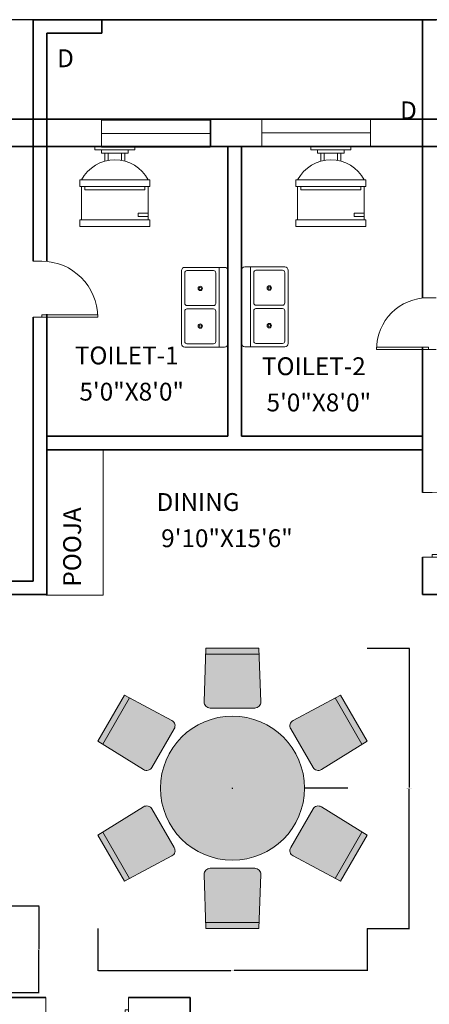
# Model space of a CAD drawing. Units: millimetres. Extents: x 27017497 to 27018854, y 7058029 to 7059154.
# Tile 47 of 91: x 27017750 to 27017886, y 7058297 to 7058623. Entities that reach past the tile are written whole.
import ezdxf

# ---------------------------------------------------------------- set-up
doc = ezdxf.new("R2010")
doc.units = ezdxf.units.MM
for name, color, linetype, lineweight in [('A-ANNO-DIMS', 2, 'Continuous', 18), ('A-ANNO-IDEN', 7, 'Continuous', 18), ('A-AREA-IDEN', 7, 'Continuous', 18), ('A-DOOR', 4, 'Continuous', 20), ('A-FLOR-CASE', 8, 'Continuous', 20), ('A-FLOR-FIXT', 9, 'Continuous', 18), ('A-FURN', 8, 'Continuous', 18), ('A-GLAZ', 4, 'Continuous', 18), ('A-WALL', 7, 'Continuous', 35)]:
    doc.layers.add(name, color=color, linetype=linetype, lineweight=lineweight)
doc.layers.add('A-FURN-PATT', color=177, linetype='Continuous', lineweight=13, true_color=0x293189)
doc.styles.get("Standard").update_dxf_attribs({"font": 'arial.ttf'})
doc.dimstyles.get("Standard").update_dxf_attribs({"dimtxt": 0.18, "dimasz": 0.18, "dimexe": 0.18, "dimexo": 0.0625, "dimgap": 0.09, "dimtad": 0, "dimtih": 1, "dimtoh": 1, "dimdec": 4, "dimzin": 0, "dimdsep": 46, "dimtxsty": 'Standard', "dimcen": 0.09, "dimadec": 0, "dimazin": 0, "dimtfac": 1, "dimtdec": 4, "dimtofl": 0, "dimtmove": 0, "dimatfit": 3, "dimfxl": 1, "dimtolj": 1, "dimtzin": 0, "dimarcsym": 0})

# ---------------------------------------------------------------- blocks, each defined once
blk = doc.blocks.new('*U2')
for p, q in [((0, 0), (0, -6)), ((40, 0), (40, -6))]:
    blk.add_line(p, q)
blk.add_lwpolyline([(0, 0), (0, 40), (1.75, 40), (1.75, 0)], close=True)
blk.add_arc((0, 0), 40, 0, 90)
blk = doc.blocks.new('6 Person Round 01')
for points in [[(-235.8, 1886.7), (-220.8, 2335), (220.8, 2335), (235.8, 1886.7, -0.424007), (185.8, 1835), (-185.8, 1835, -0.424007)], [(-740.7, 1322.9), (-1121.5, 1560), (-900.7, 1942.5), (-504.9, 1731.3, -0.424007), (-485.2, 1662.2), (-671, 1340.3, -0.424007)], [(504.9, 1731.3), (900.7, 1942.5), (1121.5, 1560), (740.7, 1322.9, -0.424007), (671, 1340.3), (485.2, 1662.2, -0.424007)], [(-504.9, 603.7), (-900.7, 392.5), (-1121.5, 775), (-740.7, 1012.1, -0.424007), (-671, 994.7), (-485.2, 672.8, -0.424007)], [(740.7, 1012.1), (1121.5, 775), (900.7, 392.5), (504.9, 603.7, -0.424007), (485.2, 672.8), (671, 994.7, -0.424007)], [(235.8, 448.3), (220.8, 0), (-220.8, 0), (-235.8, 448.3, -0.424007), (-185.8, 500), (185.8, 500, -0.424007)]]:
    blk.add_lwpolyline(points, format="xyb", close=True)
for points in [[(222.5, 2285), (-222.5, 2285)], [(-856.5, 1918.9), (-1079, 1533.6)], [(1079, 1533.6), (856.5, 1918.9)], [(-1079, 801.4), (-856.5, 416.1)], [(856.5, 416.1), (1079, 801.4)], [(-222.5, 50), (222.5, 50)]]:
    blk.add_lwpolyline(points)
blk.add_circle((0, 1167.5), 600)
blk = doc.blocks.new('*U6')
for p, q in [((-10, 22), (-10, 12)), ((-10, 21), (-7, 21)), ((-7, 21), (-7, 20)), ((10, 12), (10, 22)), ((-7, 20), (-10, 20)), ((10.5, 12), (-10.5, 12)), ((-10.5, 10), (-10.5, 12)), ((9, 13), (-9, 13)), ((-9, 13), (-9, 12)), ((9, 12), (9, 13)), ((10.5, 12), (10.5, 10)), ((10.5, 10), (-10.5, 10)), ((-3, 4.4065), (-3, 2)), ((-2, 2), (-2, 4.1658)), ((2, 4.1658), (2, 2)), ((3, 2), (3, 4.4065)), ((4, 2), (-4, 2)), ((-4, 2), (-4, 1)), ((4, 1), (4, 2))]:
    blk.add_line(p, q)
for points in [[(10.5, 22), (10.5, 24), (-10.5, 24), (-10.5, 22)], [(6, 0), (6, 1), (-6, 1), (-6, 0)]]:
    blk.add_lwpolyline(points, close=True)
blk.add_arc((0, 15.3333), 11.3333, 208.0725, 331.9275)
blk = doc.blocks.new('Sink-double - 36 in top')
for p, q in [((-18, -4), (18, -4)), ((-0.75, -18.5), (-0.75, -6.5)), ((0.75, -6.5), (0.75, -18.5))]:
    blk.add_line(p, q)
for points in [[(-16.5, 0), (16.5, 0)], [(-18, -19.5), (-18, -1.5)], [(18, -1.5), (18, -19.5)], [(-16.5, -18.5), (-16.5, -6.5)], [(-15.5, -5.5), (-1.75, -5.5)], [(1.75, -5.5), (15.5, -5.5)], [(16.5, -6.5), (16.5, -18.5)], [(16.5, -21), (-16.5, -21)], [(-1.75, -19.5), (-15.5, -19.5)], [(15.5, -19.5), (1.75, -19.5)]]:
    blk.add_lwpolyline(points)
for centre, radius in [((-8.5, -12.5), 1), ((-8.5, -12.5), 0.5), ((8.5, -12.5), 1), ((8.5, -12.5), 0.5)]:
    blk.add_circle(centre, radius)
for centre, radius, start, end in [((-16.5, -1.5), 1.5, 90, 180), ((16.5, -1.5), 1.5, 0, 90), ((-15.5, -6.5), 1, 90, 180), ((-1.75, -6.5), 1, 0, 90), ((1.75, -6.5), 1, 90, 180), ((15.5, -6.5), 1, 0, 90), ((-16.5, -19.5), 1.5, 180, 270), ((-15.5, -18.5), 1, 180, 270), ((-1.75, -18.5), 1, 270, 0), ((1.75, -18.5), 1, 180, 270), ((15.5, -18.5), 1, 270, 0), ((16.5, -19.5), 1.5, 270, 0)]:
    blk.add_arc(centre, radius, start, end)
blk = doc.blocks.new('WINDOW-SINGLE-LIGHT')
blk.add_lwpolyline([(36, 4.5), (36, 0), (0, 0), (0, 9), (36, 9), (36, 4.5), (0, 4.5)])
blk = doc.blocks.new('*D35')
at = {"layer": 'A-ANNO-DIMS', "color": 0, "lineweight": -2, "transparency": 16777216}
for p, q in [((27017865.35, 7058414.72), (27017879.4, 7058414.72)), ((27017879.22, 7058414.54), (27017879.22, 7058368.46)), ((27017879.22, 7058322.01), (27017879.22, 7058368.09)), ((27017865.35, 7058321.83), (27017879.4, 7058321.83))]:
    blk.add_line(p, q, dxfattribs=at)
at = {"layer": 'A-ANNO-DIMS', "color": 0, "transparency": 16777216}
for points in [[(27017879.19, 7058414.54), (27017879.25, 7058414.54), (27017879.22, 7058414.72)], [(27017879.19, 7058322.01), (27017879.25, 7058322.01), (27017879.22, 7058321.83)]]:
    blk.add_solid(points, dxfattribs=at)
at = {"layer": 'Defpoints', "color": 0, "transparency": 16777216}
for p in [(27017865.29, 7058414.72), (27017879.22, 7058414.72), (27017865.29, 7058321.83)]:
    blk.add_point(p, dxfattribs=at)
at = {"layer": 'A-ANNO-DIMS', "color": 0, "transparency": 16777216, "insert": (27017879.22, 7058368.28), "char_height": 0.18, "attachment_point": 5}
blk.add_mtext('\\A1;DINING SET 93 TYP.', dxfattribs=at)
blk = doc.blocks.new('*D36')
at = {"layer": 'A-ANNO-DIMS', "color": 0, "lineweight": -2, "transparency": 16777216}
for p, q in [((27017776.05, 7058321.77), (27017776.05, 7058307.71)), ((27017865.29, 7058321.77), (27017865.29, 7058307.71)), ((27017776.23, 7058307.89), (27017820.14, 7058307.89)), ((27017865.11, 7058307.89), (27017821.2, 7058307.89))]:
    blk.add_line(p, q, dxfattribs=at)
at = {"layer": 'A-ANNO-DIMS', "color": 0, "transparency": 16777216}
for points in [[(27017776.23, 7058307.92), (27017776.23, 7058307.86), (27017776.05, 7058307.89)], [(27017865.11, 7058307.92), (27017865.11, 7058307.86), (27017865.29, 7058307.89)]]:
    blk.add_solid(points, dxfattribs=at)
at = {"layer": 'Defpoints', "color": 0, "transparency": 16777216}
for p in [(27017776.05, 7058321.83), (27017865.29, 7058321.83), (27017865.29, 7058307.89)]:
    blk.add_point(p, dxfattribs=at)
at = {"layer": 'A-ANNO-DIMS', "color": 0, "transparency": 16777216, "insert": (27017820.67, 7058307.89), "char_height": 0.18, "attachment_point": 5}
blk.add_mtext('\\A1;89 TYP.', dxfattribs=at)
blk = doc.blocks.new('*D40')
at = {"layer": 'A-ANNO-DIMS', "color": 0, "lineweight": -2, "transparency": 16777216}
for p, q in [((27017746.33, 7058329.26), (27017756.63, 7058329.26)), ((27017756.45, 7058329.08), (27017756.45, 7058315.09)), ((27017756.45, 7058300.72), (27017756.45, 7058314.72)), ((27017746.33, 7058300.54), (27017756.63, 7058300.54))]:
    blk.add_line(p, q, dxfattribs=at)
at = {"layer": 'A-ANNO-DIMS', "color": 0, "transparency": 16777216}
for points in [[(27017756.42, 7058329.08), (27017756.48, 7058329.08), (27017756.45, 7058329.26)], [(27017756.42, 7058300.72), (27017756.48, 7058300.72), (27017756.45, 7058300.54)]]:
    blk.add_solid(points, dxfattribs=at)
at = {"layer": 'Defpoints', "color": 0, "transparency": 16777216}
for p in [(27017746.26, 7058329.26), (27017756.45, 7058329.26), (27017746.26, 7058300.54)]:
    blk.add_point(p, dxfattribs=at)
at = {"layer": 'A-ANNO-DIMS', "color": 0, "transparency": 16777216, "insert": (27017756.45, 7058314.9), "char_height": 0.18, "attachment_point": 5}
blk.add_mtext('\\A1;29 TYP.', dxfattribs=at)
blk = doc.blocks.new('*D48')
at = {"layer": 'A-ANNO-DIMS', "color": 0, "lineweight": -2, "transparency": 16777216}
for p, q in [((27018463.5, 7058622.91), (27017497.54, 7058622.91)), ((27017497.72, 7058622.73), (27017497.72, 7058357.75)), ((27017497.72, 7058092.41), (27017497.72, 7058357.39)), ((27018555.13, 7058092.23), (27017497.54, 7058092.23))]:
    blk.add_line(p, q, dxfattribs=at)
at = {"layer": 'A-ANNO-DIMS', "color": 0, "transparency": 16777216}
for points in [[(27017497.69, 7058622.73), (27017497.75, 7058622.73), (27017497.72, 7058622.91)], [(27017497.69, 7058092.41), (27017497.75, 7058092.41), (27017497.72, 7058092.23)]]:
    blk.add_solid(points, dxfattribs=at)
at = {"layer": 'Defpoints', "color": 0, "transparency": 16777216}
for p in [(27018463.56, 7058622.91), (27017497.72, 7058092.23), (27018555.19, 7058092.23)]:
    blk.add_point(p, dxfattribs=at)
at = {"layer": 'A-ANNO-DIMS', "color": 0, "transparency": 16777216, "insert": (27017497.72, 7058357.57), "char_height": 0.18, "attachment_point": 5}
blk.add_mtext('\\A1;530.7', dxfattribs=at)
blk = doc.blocks.new('*D54')
at = {"layer": 'A-ANNO-DIMS', "color": 0, "lineweight": -2, "transparency": 16777216}
for p, q in [((27017820.58, 7058368.28), (27017820.76, 7058368.28)), ((27017820.67, 7058368.19), (27017820.67, 7058368.37)), ((27017858.86, 7058368.27), (27017844.72, 7058368.27))]:
    blk.add_line(p, q, dxfattribs=at)
at = {"layer": 'A-ANNO-DIMS', "color": 0, "transparency": 16777216}
blk.add_solid([(27017844.72, 7058368.3), (27017844.72, 7058368.24), (27017844.54, 7058368.27)], dxfattribs=at)
at = {"layer": 'Defpoints', "color": 0, "transparency": 16777216}
for p in [(27017796.8, 7058368.28), (27017844.54, 7058368.27)]:
    blk.add_point(p, dxfattribs=at)
at = {"layer": 'A-ANNO-DIMS', "color": 0, "transparency": 16777216, "insert": (27017859.54, 7058368.27), "char_height": 0.18, "attachment_point": 5}
blk.add_mtext('\\A1;2X ∅47.74', dxfattribs=at)

msp = doc.modelspace()

# ---------------------------------------------------------------- hatches: boundary and pattern name
at = {"layer": 'A-FURN-PATT'}
h = msp.add_hatch(color=256, dxfattribs=at)
h.dxf.hatch_style = 1
h.paths.add_polyline_path([(27017801.368, 7058387.955, 0.4240071), (27017800.582, 7058390.704), (27017786.594, 7058398.17), (27017777.742, 7058382.838), (27017791.202, 7058374.457, 0.4240071), (27017793.976, 7058375.151)])
h.paths.add_polyline_path([(27017829.522, 7058412.733), (27017811.818, 7058412.733), (27017811.29, 7058396.886, 0.4240071), (27017813.278, 7058394.831), (27017828.062, 7058394.831, 0.4240071), (27017830.05, 7058396.886)])
h.paths.add_polyline_path([(27017793.976, 7058361.399, 0.4240071), (27017791.202, 7058362.093), (27017777.742, 7058353.712), (27017786.594, 7058338.38), (27017800.582, 7058345.846, 0.4240071), (27017801.368, 7058348.596)])
h.paths.add_polyline_path([(27017830.05, 7058339.664, 0.4240071), (27017828.062, 7058341.72), (27017813.278, 7058341.72, 0.4240071), (27017811.29, 7058339.664), (27017811.818, 7058323.817), (27017829.522, 7058323.817)])
h.paths.add_polyline_path([(27017863.598, 7058353.712), (27017850.138, 7058362.093, 0.4240071), (27017847.364, 7058361.399), (27017839.972, 7058348.596, 0.4240071), (27017840.758, 7058345.846), (27017854.746, 7058338.38)])
h.paths.add_polyline_path([(27017854.746, 7058398.17), (27017840.758, 7058390.704, 0.4240071), (27017839.972, 7058387.955), (27017847.364, 7058375.151, 0.4240071), (27017850.138, 7058374.457), (27017863.598, 7058382.838)])
h.paths.add_polyline_path([(27017856.502, 7058399.107), (27017854.746, 7058398.17), (27017863.598, 7058382.838), (27017865.287, 7058383.89)])
h.paths.add_polyline_path([(27017829.455, 7058414.723), (27017811.884, 7058414.723), (27017811.818, 7058412.733), (27017829.522, 7058412.733)])
h.paths.add_polyline_path([(27017786.594, 7058398.17), (27017784.838, 7058399.107), (27017776.052, 7058383.89), (27017777.742, 7058382.838)])
h.paths.add_polyline_path([(27017777.742, 7058353.712), (27017776.052, 7058352.66), (27017784.838, 7058337.443), (27017786.594, 7058338.38)])
h.paths.add_polyline_path([(27017829.522, 7058323.817), (27017811.818, 7058323.817), (27017811.884, 7058321.828), (27017829.455, 7058321.828)])
h.paths.add_polyline_path([(27017865.287, 7058352.66), (27017863.598, 7058353.712), (27017854.746, 7058338.38), (27017856.502, 7058337.443)])
h = msp.add_hatch(color=256, dxfattribs=at)
h.dxf.hatch_style = 1
h.paths.add_polyline_path([(27017796.8, 7058368.275, 1), (27017844.54, 7058368.275, 1)])

# ---------------------------------------------------------------- linework, layer by layer
at = {"layer": 'A-FLOR-CASE'}
for p, q in [((27017777.868, 7058432.276), (27017777.868, 7058480.412)), ((27017758.882, 7058432.276), (27017777.868, 7058432.276))]:
    msp.add_line(p, q, dxfattribs=at)
at = {"layer": 'A-GLAZ'}
msp.add_lwpolyline([(27017813.45, 7058589.881), (27017830.412, 7058589.881), (27017830.412, 7058580.963), (27017813.45, 7058580.963)], close=True, dxfattribs=at)
at = {"layer": 'A-WALL'}
for p, q in [((27017754.666, 7058589.912), (27017754.666, 7058622.912)), ((27017754.666, 7058622.912), (27017777.344, 7058622.912)), ((27017777.344, 7058622.912), (27017888.211, 7058622.912)), ((27017777.344, 7058618.412), (27017777.344, 7058622.912)), ((27017883.666, 7058622.912), (27017883.666, 7058530.724)), ((27017759.166, 7058589.912), (27017759.166, 7058618.412)), ((27017759.166, 7058618.412), (27017777.344, 7058618.412)), ((27017613.666, 7058589.912), (27018310.606, 7058589.912)), ((27017754.666, 7058589.912), (27017754.666, 7058542.877)), ((27017759.166, 7058589.912), (27017759.166, 7058543.053)), ((27017622.666, 7058580.912), (27018223.606, 7058580.912)), ((27017819.166, 7058580.912), (27017819.166, 7058484.912)), ((27017823.666, 7058580.912), (27017823.666, 7058484.912)), ((27017754.666, 7058524.331), (27017754.666, 7058436.912)), ((27017759.166, 7058525.375), (27017759.166, 7058432.412)), ((27017883.666, 7058514.376), (27017883.666, 7058466.205)), ((27017759.166, 7058484.912), (27017819.166, 7058484.912)), ((27017823.666, 7058484.912), (27017883.666, 7058484.912)), ((27017759.166, 7058480.412), (27017819.166, 7058480.412)), ((27017819.166, 7058480.412), (27017883.666, 7058480.412)), ((27017883.666, 7058444.814), (27017883.666, 7058432.412)), ((27017743.085, 7058436.912), (27017754.666, 7058436.912)), ((27017744.287, 7058432.412), (27017759.166, 7058432.412)), ((27017883.666, 7058432.412), (27018041.166, 7058432.412)), ((27017743.666, 7058298.912), (27017758.779, 7058298.912)), ((27017786.261, 7058298.912), (27017806.666, 7058298.912)), ((27017806.666, 7058298.912), (27017806.666, 7058243.912))]:
    msp.add_line(p, q, dxfattribs=at)

# ---------------------------------------------------------------- block references
at = {"layer": 'A-DOOR'}
for p, xscale, yscale, zscale, rotation in [((27017757.448, 7058524.331), -0.4636703714562217, 0.4636703714562217, 0.4636703714562217, 270), ((27017885.592, 7058513.597), 0.4301822298564029, 0.4301822298564029, 0.4301822298564029, 90.00000000000003), ((27017886.848, 7058444.814), -0.5347783892510444, 0.5347783892510444, 0.5347783892510444, 270), ((27017786.261, 7058294.793), 0.6870473523349573, 0.6870473523349573, 0.6870473523349573, 180)]:
    msp.add_blockref('*U2', p, dxfattribs=dict(at, xscale=xscale, yscale=yscale, zscale=zscale, rotation=rotation))
at = {"layer": 'A-FLOR-FIXT'}
for name, p, xscale, yscale, zscale, rotation in [('*U6', (27017781.714, 7058580.878), 1.105119395603938, 1.105119395603938, 1.105119395603938, 180), ('*U6', (27017853.324, 7058580.908), 1.105119395603938, 1.105119395603938, 1.105119395603938, 180), ('Sink-double - 36 in top', (27017819.18, 7058527.641), -0.7340308267416257, 0.7340308267416257, 0.7340308267416257, 270), ('Sink-double - 36 in top', (27017823.7, 7058527.759), 0.7340308267416257, 0.7340308267416257, 0.7340308267416257, 89.99999999999999)]:
    msp.add_blockref(name, p, dxfattribs=dict(at, xscale=xscale, yscale=yscale, zscale=zscale, rotation=rotation))
at = {"layer": 'A-FURN', "xscale": 0.0397836222497725, "yscale": 0.0397836222497725, "zscale": 0.0397836222497725}
msp.add_blockref('6 Person Round 01', (27017820.67, 7058321.828), dxfattribs=at)
at = {"layer": 'A-GLAZ'}
for p in [(27017777.291, 7058580.67), (27017830.425, 7058580.903)]:
    msp.add_blockref('WINDOW-SINGLE-LIGHT', p, dxfattribs=at)

# ---------------------------------------------------------------- texts
at = {"layer": 'A-ANNO-DIMS'}
for s, height, p in [('5\'0"X8\'0"', 5.9118, (27017769.945, 7058496.704)), ('5\'0"X8\'0"', 5.9118, (27017831.968, 7058493.134)), ('9\'10"X15\'6"', 5.91176, (27017797.042, 7058448.139))]:
    msp.add_text(s, height=height, dxfattribs=at).set_placement(p)
at = {"layer": 'A-ANNO-IDEN'}
for p in [(27017762.55, 7058607.171), (27017876.23, 7058589.912)]:
    msp.add_text('D', height=5.912, rotation=360, dxfattribs=at).set_placement(p)
at = {"layer": 'A-AREA-IDEN'}
for s, p in [('TOILET-1', (27017768.41, 7058508.701)), ('TOILET-2', (27017830.433, 7058505.131)), ('DINING', (27017795.506, 7058460.137))]:
    msp.add_text(s, height=5.9118, dxfattribs=at).set_placement(p)
msp.add_text('POOJA', height=5.9118, rotation=90, dxfattribs=at).set_placement((27017770.478, 7058435.06))

# ---------------------------------------------------------------- dimensions: what is measured, and where the dimension line sits
at = {"layer": 'A-ANNO-DIMS'}
dim = msp.add_linear_dim(base=(27017497.716, 7058092.23), p1=(27018463.561, 7058622.912), p2=(27018555.192, 7058092.23), angle=90, dimstyle='Standard', override={"dimdec": 1, "dimlfac": 1, "dimrnd": 0, "dimzin": 0, "dimdsep": 46, "dimlunit": 2}, dxfattribs=at)
dim.commit()
dim.dimension.update_dxf_attribs({"geometry": '*D48', "text_midpoint": (27017497.716, 7058357.571)})
for base, p1, p2, text, picture, middle in [((27017879.221, 7058414.723), (27017865.287, 7058321.828), (27017865.287, 7058414.723), 'DINING SET <> TYP.', '*D35', (27017879.221, 7058368.275)), ((27017756.445, 7058329.264), (27017746.263, 7058300.544), (27017746.263, 7058329.264), '<> TYP.', '*D40', (27017756.445, 7058314.904))]:
    dim = msp.add_linear_dim(base=base, p1=p1, p2=p2, angle=90, text=text, dimstyle='Standard', override={"dimdec": 0, "dimlfac": 1, "dimrnd": 0, "dimzin": 0, "dimdsep": 46, "dimlunit": 2}, dxfattribs=at)
    dim.commit()
    dim.dimension.update_dxf_attribs({"geometry": picture, "text_midpoint": middle})
dim = msp.add_diameter_dim_2p(p1=(27017796.8, 7058368.276), p2=(27017844.54, 7058368.275), text='2X <>', dimstyle='Standard', override={"dimdec": 2, "dimlfac": 1, "dimrnd": 0, "dimzin": 0, "dimdsep": 46, "dimlunit": 2}, dxfattribs=at)
dim.commit()
dim.dimension.update_dxf_attribs({"geometry": '*D54', "text_midpoint": (27017858.862, 7058368.275), "dimtype": 163})
dim = msp.add_linear_dim(base=(27017865.287, 7058307.894), p1=(27017776.052, 7058321.828), p2=(27017865.287, 7058321.828), text='<> TYP.', dimstyle='Standard', override={"dimdec": 0, "dimlfac": 1, "dimrnd": 0, "dimzin": 0, "dimdsep": 46, "dimlunit": 2}, dxfattribs=at)
dim.commit()
dim.dimension.update_dxf_attribs({"geometry": '*D36', "text_midpoint": (27017820.67, 7058307.894)})

doc.saveas('drawing.dxf')
